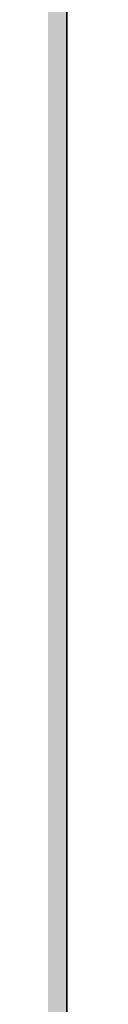
# Model space of a CAD drawing. Units: inches. Extents: x 2083 to 3317, y 1141 to 2115.
# Tile 170 of 256: x 3126.959687 to 3126.959831, y 1263.265937 to 1263.274018. Entities that reach past the tile are written whole.
import ezdxf

# ---------------------------------------------------------------- set-up
doc = ezdxf.new("R2010")
doc.units = ezdxf.units.IN
doc.layers.add('A-ANNO-DIMS', color=2, linetype='Continuous', lineweight=18)
doc.layers.add('A-WALL', color=7, linetype='Continuous', lineweight=35)
doc.layers.add('A-WALL-PATT', color=251, linetype='Continuous', lineweight=13, true_color=0x636466)
doc.styles.get("Standard").update_dxf_attribs({"font": 'arial.ttf'})
doc.dimstyles.new('ISO-25', dxfattribs={"dimtxt": 12, "dimasz": 12, "dimexe": 1.25, "dimexo": 0.625, "dimtad": 1, "dimlunit": 3, "dimtxsty": 'Standard', "dimcen": 2.5, "dimadec": 0, "dimazin": 0, "dimtfac": 1, "dimtmove": 0, "dimatfit": 3, "dimfxl": 1, "dimarcsym": 0})

# ---------------------------------------------------------------- blocks, each defined once
blk = doc.blocks.new('*D9')
at = {"layer": 'A-ANNO-DIMS', "color": 0, "lineweight": -2, "transparency": 16777216}
for p, q in [((3127.5847832, 1486.7613601), (3190.4030896, 1486.7613601)), ((3189.1530896, 1474.7613601), (3189.1530896, 1275.2613601)), ((3127.5847832, 1263.2613601), (3190.4030896, 1263.2613601))]:
    blk.add_line(p, q, dxfattribs=at)
at = {"layer": 'A-ANNO-DIMS', "color": 0, "transparency": 16777216}
for points in [[(3187.1530896, 1474.7613601), (3191.1530896, 1474.7613601), (3189.1530896, 1486.7613601)], [(3187.1530896, 1275.2613601), (3191.1530896, 1275.2613601), (3189.1530896, 1263.2613601)]]:
    blk.add_solid(points, dxfattribs=at)
at = {"layer": 'Defpoints', "color": 0, "transparency": 16777216}
for p in [(3126.9597832, 1486.7613601), (3126.9597832, 1263.2613601), (3189.1530896, 1263.2613601)]:
    blk.add_point(p, dxfattribs=at)
at = {"layer": 'A-ANNO-DIMS', "color": 0, "transparency": 16777216, "insert": (3182.4012138, 1375.0113601), "char_height": 12, "attachment_point": 5, "rotation": 90}
blk.add_mtext('18\'-7.5"', dxfattribs=at)

msp = doc.modelspace()

# ---------------------------------------------------------------- hatches: boundary and pattern name
at = {"layer": 'A-WALL-PATT'}
h = msp.add_hatch(color=256, dxfattribs=at)
h.dxf.hatch_style = 1
h.paths.add_polyline_path([(3126.9597832, 2020.7613601), (2748.9597832, 2020.7613601), (2604.9597832, 2020.7613601), (2226.9597832, 2020.7613601), (2226.9597832, 1702.7613601), (2466.9597832, 1702.7613601), (2466.9597832, 1582.7613601), (2418.9597832, 1582.7613601), (2418.9597832, 1477.7613601), (2226.9597832, 1477.7613601), (2226.9597832, 1263.2613601), (2544.9597832, 1263.2613601), (2544.9597832, 1411.7613601), (2604.9597832, 1411.7613601), (2685.9597832, 1411.7613601), (2685.9597832, 1420.7613601), (2604.9597832, 1420.7613601), (2604.9597832, 1573.7613601), (2604.9597832, 1702.7613601), (2604.9597832, 2011.7613601), (2748.9597832, 2011.7613601), (2748.9597832, 1702.7613601), (2862.9597832, 1702.7613601), (2862.9597832, 1621.7613601), (2871.9597832, 1621.7613601), (2871.9597832, 1702.7613601), (2883.9597832, 1702.7613601), (2883.9597832, 1706.9394595, -0.026459), (2883.9597832, 1711.7613601), (2757.9597832, 1711.7613601), (2757.9597832, 1807.7613601), (2787.9597832, 1807.7613601), (2787.9597832, 1812.2613601), (2757.9597832, 1812.2613601), (2757.9597832, 2011.7613601), (2877.9597832, 2011.7613601), (2877.9597832, 1812.2613601), (2847.9597832, 1812.2613601), (2847.9597832, 1807.7613601), (2889.8357425, 1807.7613601), (2889.8357425, 1812.2613601), (2882.4597832, 1812.2613601), (2882.4597832, 2011.7613601), (3117.9597832, 2011.7613601), (3117.9597832, 1812.2613601), (2937.8357425, 1812.2613601), (2937.8357425, 1807.7613601), (2995.7097832, 1807.7613601), (2995.7097832, 1796.1176655), (3000.2097832, 1796.1176655), (3000.2097832, 1807.7613601), (3117.9597832, 1807.7613601), (3117.9597832, 1711.7613601), (3000.2097832, 1711.7613601), (3000.2097832, 1760.1176655), (2998.5727047, 1760.1176655, -0.020711), (2995.7097832, 1760.1176655), (2995.7097832, 1711.7613601), (2931.9597832, 1711.7613601), (2931.9597832, 1702.7613601), (3126.9597832, 1702.7613601)])
h.paths.add_polyline_path([(2471.4597832, 2011.7613601), (2471.4597832, 1810.0113601), (2462.7169357, 1810.0113601), (2462.7169357, 1805.5113601), (2505.9597832, 1805.5113601), (2505.9597832, 1810.0113601), (2475.9597832, 1810.0113601), (2475.9597832, 2011.7613601), (2595.9597832, 2011.7613601), (2595.9597832, 1810.0113601), (2565.9597832, 1810.0113601), (2565.9597832, 1805.5113601), (2595.9597832, 1805.5113601), (2595.9597832, 1711.7613601), (2235.9597832, 1711.7613601), (2235.9597832, 1805.5113601), (2353.7097832, 1805.5113601), (2353.7097832, 1796.0541624), (2358.2097832, 1796.0541624), (2358.2097832, 1805.5113601), (2414.7169357, 1805.5113601), (2414.7169357, 1810.0113601), (2235.9597832, 1810.0113601), (2235.9597832, 2011.7613601)], flags=16)
h.paths.add_polyline_path([(2270.2047343, 1994.6100082), (2270.2047343, 1970.6100082), (2246.2047343, 1970.6100082), (2246.2047343, 1994.6100082)], flags=0)
edge = h.paths.add_edge_path(flags=0)
edge.add_ellipse((2332.027391, 1899.7981761), major_axis=(-3.0429938, 3.0429938), ratio=0.16825245, start_angle=-161.3321656, end_angle=-156.3071136, ccw=False)
edge.add_ellipse((2333.0820373, 1898.7435297), major_axis=(-1.0546463, 1.0546463), ratio=0.453532097, start_angle=-123.371019, end_angle=-94.1591066)
edge = h.paths.add_edge_path(flags=0)
edge.add_ellipse((2332.027391, 1968.8762897), major_axis=(3.0429938, 3.0429938), ratio=0.16825245, start_angle=18.6678344, end_angle=23.6928864)
edge.add_spline(control_points=[(2332.9255964, 1970.6911045), (2332.2267681, 1970.3360997), (2330.8937087, 1969.6589054), (2328.4130803, 1970.9321376), (2327.2039345, 1967.7487119), (2324.7095965, 1969.9555886), (2322.5328223, 1967.012354), (2320.0128462, 1971.2958124), (2317.6803077, 1968.1578449), (2316.0405263, 1967.1020468), (2315.4269045, 1966.8096022)], knot_values=[0, 0, 0, 0, 2.267059, 4.324559, 6.685584, 8.878641, 11.121502, 14.300359, 17.755284, 19.732645, 19.732645, 19.732645, 19.732645], degree=3, periodic=0)
edge.add_ellipse((2332.027391, 1968.8762897), major_axis=(3.0429938, 3.0429938), ratio=0.16825245, start_angle=18.6678344, end_angle=23.6928864, ccw=False)
edge.add_ellipse((2333.0820373, 1969.930936), major_axis=(1.0546463, 1.0546463), ratio=0.453532097, start_angle=56.628981, end_angle=85.8408934, ccw=False)
edge = h.paths.add_edge_path(flags=0)
edge.add_spline(control_points=[(2296.4282874, 1967.9879081), (2293.6278045, 1965.3363137), (2287.7036238, 1959.727094), (2299.7438601, 1949.9956993), (2294.5325909, 1935.6685275), (2290.5732281, 1920.6035119), (2293.3941244, 1909.9736911), (2296.1854073, 1904.9665431)], knot_values=[0.099185, 0.099185, 0.099185, 0.099185, 0.345301, 0.619822, 0.982653, 1.386093, 1.810555, 1.810555, 1.810555, 1.810555], degree=3, periodic=0)
edge.add_spline(control_points=[(2296.1854073, 1904.9665431), (2297.3835817, 1902.6193002), (2298.0009694, 1901.9493116), (2298.5529698, 1901.4681549)], knot_values=[0.006246, 0.006246, 0.006246, 0.006246, 0.055476, 0.055476, 0.055476, 0.055476], degree=3, periodic=0)
edge.add_spline(control_points=[(2298.5529698, 1901.4681549), (2297.2586121, 1900.9232238), (2295.2252939, 1900.2321257), (2293.0602287, 1900.6142053), (2292.1014227, 1900.788415), (2292.0895776, 1900.790568)], knot_values=[0.312835, 0.312835, 0.312835, 0.312835, 0.40178, 0.474987, 0.475903, 0.475903, 0.475903, 0.475903], degree=3, periodic=0)
edge.add_arc((2292.7936464, 1904.6641088), 3.9370079, 215.4208969, 259.6981795, ccw=False)
edge.add_spline(control_points=[(2289.5853139, 1902.3823039), (2289.4766524, 1902.5350874), (2289.3684805, 1902.6880353), (2289.2608648, 1902.8411699)], knot_values=[0.102872, 0.102872, 0.102872, 0.102872, 0.116896, 0.116896, 0.116896, 0.116896], degree=3, periodic=0)
edge.add_spline(control_points=[(2289.2608648, 1902.8411699), (2288.6866042, 1902.5501922), (2287.6400477, 1902.0199025), (2285.8813368, 1901.8739536), (2283.8529717, 1901.5043521), (2281.7199871, 1899.7105375), (2278.4669913, 1899.492942), (2276.1571361, 1901.8832022), (2272.2589526, 1899.8040711), (2267.7776054, 1901.8431828), (2262.2438819, 1900.1840326), (2257.414927, 1901.7820606), (2254.318374, 1900.7261196), (2253.1782849, 1900.3373431)], knot_values=[0, 0, 0, 0, 1.907977, 3.477176, 5.261074, 7.972851, 11.680248, 13.717921, 16.939592, 22.789562, 27.502503, 33.595215, 37.145618, 37.145618, 37.145618, 37.145618], degree=3, periodic=0)
edge.add_line((2253.1782849, 1900.3373431), (2250.2442397, 1902.8411699))
edge.add_line((2250.2442397, 1902.8411699), (2250.2442397, 1965.8332959))
edge.add_line((2250.2442397, 1965.8332959), (2253.1782849, 1968.3371226))
edge.add_spline(control_points=[(2253.1782849, 1968.3371226), (2254.318374, 1967.9483462), (2257.414927, 1966.8924051), (2262.2438819, 1968.4904332), (2267.7776054, 1966.8312829), (2271.5267301, 1968.5372172), (2273.8759143, 1967.8282895), (2274.2067012, 1967.7276424)], knot_values=[0, 0, 0, 0, 0.09018, 0.244935, 0.364644, 0.513233, 0.537855, 0.537855, 0.537855, 0.537855], degree=3, periodic=0)
edge.add_arc((2274.3528869, 1963.7933495), 3.9370079, 72.0511336, 92.1279492, ccw=False)
edge.add_arc((2281.2969331, 1985.2300027), 18.5962982, 252.05113361, 288.56572166)
edge.add_arc((2292.3167172, 1956.0288805), 12.6460805, 71.02678788, 113.77821843, ccw=False)
edge = h.paths.add_edge_path(flags=0)
edge.add_spline(control_points=[(2274.8994147, 1951.8561946), (2275.066156, 1951.6165924), (2275.2326866, 1951.3765878), (2275.3979871, 1951.1358545)], knot_values=[1.409916, 1.409916, 1.409916, 1.409916, 1.43159, 1.43159, 1.43159, 1.43159], degree=3, periodic=0)
edge.add_spline(control_points=[(2275.3979871, 1951.1358545), (2275.7921055, 1950.5618854), (2276.1792311, 1949.9837745), (2276.5455462, 1949.3971029)], knot_values=[1.358238, 1.358238, 1.358238, 1.358238, 1.409916, 1.409916, 1.409916, 1.409916], degree=3, periodic=0)
edge.add_line((2276.5455462, 1949.3971029), (2277.437289, 1947.8621847))
edge.add_spline(control_points=[(2277.437289, 1947.8621847), (2276.3038341, 1945.6731147), (2274.6396979, 1942.4268817), (2274.631615, 1938.0938998), (2272.7991237, 1930.8515498), (2274.3564261, 1943.8970461), (2275.9476814, 1947.9233558), (2276.5455462, 1949.3971029)], knot_values=[0.005632, 0.005632, 0.005632, 0.005632, 0.186014, 0.266002, 0.357087, 0.59639, 0.739732, 0.739732, 0.739732, 0.739732], degree=3, periodic=0)
edge.add_spline(control_points=[(2276.5455462, 1949.3971029), (2276.1792311, 1949.9837745), (2275.7921055, 1950.5618854), (2275.3979871, 1951.1358545)], knot_values=[1.358238, 1.358238, 1.358238, 1.358238, 1.409916, 1.409916, 1.409916, 1.409916], degree=3, periodic=0)
edge.add_spline(control_points=[(2275.3979871, 1951.1358545), (2274.9425002, 1950.0804523), (2274.2077604, 1948.0252718), (2273.9346018, 1944.8514774), (2272.4685341, 1937.6274891), (2273.4662155, 1945.6964663), (2274.7006154, 1951.0594725), (2274.8994147, 1951.8561946)], knot_values=[0.104364, 0.104364, 0.104364, 0.104364, 0.189636, 0.269624, 0.36071, 0.600013, 0.644622, 0.644622, 0.644622, 0.644622], degree=3, periodic=0)
h.paths.add_polyline_path([(2269.1675139, 1963.1275729, -0.357527), (2268.170633, 1960.9763695, -0.092561), (2268.170633, 1939.4363249, -0.357527), (2269.1675139, 1937.2851215, -0.357527), (2267.0163105, 1938.2820024, -0.164785), (2254.6855813, 1938.2820024, -0.357527), (2252.5343779, 1937.2851215, -0.357527), (2253.5312587, 1939.4363249, -0.092561), (2253.5312587, 1960.9763695, -0.357527), (2252.5343779, 1963.1275729, -0.357527), (2254.6855813, 1962.130692, -0.164785), (2267.0163105, 1962.130692, -0.357527)], flags=0)
h.paths.add_polyline_path([(2248.8740679, 1967.8017998), (2248.8740679, 1957.0277095), (2249.4577833, 1957.0277095), (2249.4577833, 1911.6467562), (2248.8740679, 1911.6467562), (2248.8740679, 1900.8726659), (2246.5118632, 1900.8726659, 0.197327), (2244.1496584, 1902.4568734), (2244.1496584, 1966.2175923, 0.197327), (2246.5118632, 1967.8017998)], flags=0)
h.paths.add_polyline_path([(2269.1675139, 1931.3893442, -0.357527), (2268.170633, 1929.2381408, -0.092561), (2268.170633, 1907.6980962, -0.357527), (2269.1675139, 1905.5468928, -0.357527), (2267.0163105, 1906.5437737, -0.164785), (2254.6855813, 1906.5437737, -0.357527), (2252.5343779, 1905.5468928, -0.357527), (2253.5312587, 1907.6980962, -0.092561), (2253.5312587, 1929.2381408, -0.357527), (2252.5343779, 1931.3893442, -0.357527), (2254.6855813, 1930.3924634, -0.164785), (2267.0163105, 1930.3924634, -0.357527)], flags=0)
edge = h.paths.add_edge_path(flags=0)
edge.add_spline(control_points=[(2276.1968578, 1906.7237016), (2276.1681442, 1909.0289278), (2276.1140492, 1913.371852), (2270.5984171, 1924.9249783), (2273.9051746, 1919.0127787), (2275.9217115, 1916.2620626), (2275.4745699, 1912.4021495), (2277.2578735, 1910.3806206), (2276.6960436, 1908.2250358), (2276.6462176, 1906.8130226), (2276.6178249, 1906.0084068)], knot_values=[0, 0, 0, 0, 8.61026, 16.221274, 18.843057, 23.804898, 27.440828, 29.356102, 31.203478, 33.650687, 33.650687, 33.650687, 33.650687], degree=3, periodic=0)
edge.add_spline(control_points=[(2276.6178249, 1906.0084068), (2276.6233131, 1905.6241436), (2276.4977381, 1904.6286608), (2275.4417789, 1903.8547251), (2274.9373144, 1903.0804497), (2274.8590804, 1902.8411699)], knot_values=[0.156488, 0.156488, 0.156488, 0.156488, 0.184398, 0.231376, 0.250598, 0.250598, 0.250598, 0.250598], degree=3, periodic=0)
edge.add_line((2274.8590804, 1902.8411699), (2276.50598, 1902.8411699))
edge.add_spline(control_points=[(2276.50598, 1902.8411699), (2276.7883084, 1903.0849395), (2277.6650711, 1904.1251958), (2278.2495378, 1904.340738), (2277.6538719, 1908.5273866), (2278.15567, 1906.2278078), (2278.100464, 1905.2859484), (2278.8466748, 1904.0690054), (2277.8567853, 1903.4149482), (2277.8741909, 1902.9910497), (2277.9035616, 1902.8411699)], knot_values=[0.059574, 0.059574, 0.059574, 0.059574, 0.080753, 0.103741, 0.16972, 0.176036, 0.207137, 0.240474, 0.262341, 0.27366, 0.27366, 0.27366, 0.27366], degree=3, periodic=0)
edge.add_line((2277.9035616, 1902.8411699), (2280.0298255, 1902.8411699))
edge.add_spline(control_points=[(2280.0298255, 1902.8411699), (2279.8882214, 1903.088398), (2279.4992571, 1903.9815512), (2280.1522839, 1905.9393491), (2278.103615, 1909.6577572), (2279.7623946, 1907.185285), (2280.3279002, 1904.8748608), (2280.4851086, 1903.4895904), (2281.4632687, 1903.2494323), (2281.7583431, 1902.9364967), (2281.8340361, 1902.8411699)], knot_values=[0.013856, 0.013856, 0.013856, 0.013856, 0.034874, 0.088867, 0.107879, 0.126738, 0.158714, 0.193757, 0.217487, 0.226722, 0.226722, 0.226722, 0.226722], degree=3, periodic=0)
edge.add_spline(control_points=[(2281.8340361, 1902.8411699), (2281.7875348, 1902.8267029), (2281.6470224, 1902.7829881), (2281.3955272, 1902.85949), (2281.088077, 1902.9852418), (2280.7206826, 1903.060902), (2280.3334513, 1903.0257257), (2280.1247668, 1902.898879), (2280.0298255, 1902.8411699)], knot_values=[0, 0, 0, 0, 0.14413, 0.435517, 0.749276, 1.153046, 1.548371, 1.878348, 1.878348, 1.878348, 1.878348], degree=3, periodic=0)
edge.add_line((2280.0298255, 1902.8411699), (2277.9035616, 1902.8411699))
edge.add_spline(control_points=[(2277.9035616, 1902.8411699), (2277.892855, 1902.7958553), (2277.865396, 1902.6796374), (2277.6074793, 1902.6874828), (2277.2740503, 1902.8006999), (2276.8379209, 1902.6197745), (2276.5838074, 1902.7892611), (2276.50598, 1902.8411699)], knot_values=[0, 0, 0, 0, 0.127189, 0.326199, 0.628009, 1.24357, 1.515331, 1.515331, 1.515331, 1.515331], degree=3, periodic=0)
edge.add_line((2276.50598, 1902.8411699), (2274.8590804, 1902.8411699))
edge.add_spline(control_points=[(2274.8590804, 1902.8411699), (2274.8144367, 1902.8985868), (2274.7251297, 1903.013446), (2274.4934765, 1903.1189684), (2274.2442854, 1902.9605386), (2273.9371207, 1903.1849416), (2273.6140395, 1902.9831428), (2273.4083164, 1902.8830449), (2273.322254, 1902.8411699)], knot_values=[0, 0, 0, 0, 0.21843, 0.436957, 0.687977, 0.990379, 1.398396, 1.69185, 1.69185, 1.69185, 1.69185], degree=3, periodic=0)
edge.add_spline(control_points=[(2273.322254, 1902.8411699), (2273.6167403, 1903.445692), (2274.2739977, 1904.5382529), (2276.0272387, 1904.5737017), (2276.2069634, 1906.5836372), (2276.1968578, 1906.7237016)], knot_values=[0.012227, 0.012227, 0.012227, 0.012227, 0.059472, 0.106218, 0.134458, 0.134458, 0.134458, 0.134458], degree=3, periodic=0)
h.paths.add_polyline_path([(2270.7760538, 1897.7898284), (2270.7760538, 1873.7898284), (2246.7760538, 1873.7898284), (2246.7760538, 1897.7898284)], flags=0)
h.paths.add_polyline_path([(2353.7097832, 1760.0050593), (2353.7097832, 1760.0541624), (2358.2097832, 1760.0541624, -0.033729)], flags=0)
h.paths.add_polyline_path([(2321.8191188, 1737.5291862), (2341.9953271, 1737.5291862, -0.414214), (2343.2032727, 1736.3212406), (2343.2032727, 1721.0205964, -0.414214), (2341.9953271, 1719.8126508), (2321.8191188, 1719.8126508, -0.414214), (2320.6111732, 1721.0205964), (2320.6111732, 1736.3212406, -0.414214)], flags=0)
h.paths.add_polyline_path([(2324.2350099, 1736.3212406), (2339.5794359, 1736.3212406, -0.414214), (2341.9953271, 1733.9053494), (2341.9953271, 1725.4497302, -0.414214), (2339.5794359, 1723.033839), (2333.6805885, 1723.033839), (2333.8453172, 1722.0454666, -0.870646), (2335.4253988, 1721.8258934, -0.767327), (2333.922694, 1721.4232449), (2331.2910241, 1721.4232449, -0.767327), (2329.7883193, 1721.8258934, -0.870646), (2331.3684009, 1722.0454666), (2331.5331296, 1723.033839), (2324.2350099, 1723.033839, -0.414214), (2321.8191188, 1725.4497302), (2321.8191188, 1733.9053494, -0.414214)], flags=0)
h.paths.add_polyline_path([(2570.4837892, 1928.6154443), (2589.6837892, 1928.6154443), (2590.1688286, 1928.6154443), (2590.1688286, 1904.9933971), (2570.4837892, 1904.9933971)], flags=0)
h.paths.add_polyline_path([(2574.4473242, 1927.2638215, -1), (2572.8288357, 1927.2638215, -1)], flags=0)
h.paths.add_polyline_path([(2573.0898665, 1926.9408768), (2573.925032, 1927.7760423), (2574.1477428, 1927.5533315), (2573.3125773, 1926.718166)], flags=0)
h.paths.add_polyline_path([(2578.7790648, 1919.7296175, -1), (2571.5916632, 1919.7296175, -1)], flags=0)
h.paths.add_polyline_path([(2578.385364, 1919.7296175, -1), (2571.985364, 1919.7296175, -1)], flags=0)
h.paths.add_polyline_path([(2331.5957638, 1729.4762156, -1), (2333.6179542, 1729.4762156, -1)], flags=0)
h.paths.add_polyline_path([(2578.0342282, 1927.2638215, -1), (2576.4157396, 1927.2638215, -1)], flags=0)
h.paths.add_polyline_path([(2576.6888513, 1927.5310886), (2576.9115621, 1927.7537993), (2577.7467276, 1926.9186339), (2577.5240168, 1926.6959231)], flags=0)
h.paths.add_polyline_path([(2578.1390648, 1909.8595388, -1), (2572.2316632, 1909.8595388, -1)], flags=0)
h.paths.add_polyline_path([(2577.745364, 1909.8595388, -1), (2572.625364, 1909.8595388, -1)], flags=0)
h.paths.add_polyline_path([(2583.7977179, 1927.2638215, -1), (2582.1792294, 1927.2638215, -1)], flags=0)
h.paths.add_polyline_path([(2582.7186487, 1927.7537993), (2583.5538142, 1926.9186339), (2583.3311034, 1926.6959231), (2582.4959379, 1927.5310886)], flags=0)
h.paths.add_polyline_path([(2582.4959379, 1927.5310886), (2582.7186487, 1927.7537993), (2583.5538142, 1926.9186339), (2583.3311034, 1926.6959231)], flags=0)
h.paths.add_polyline_path([(2587.7390648, 1920.5296175, -1), (2581.8316632, 1920.5296175, -1)], flags=0)
h.paths.add_polyline_path([(2587.345364, 1920.5296175, -1), (2582.225364, 1920.5296175, -1)], flags=0)
h.paths.add_polyline_path([(2587.3846219, 1927.2638215, -1), (2585.7661333, 1927.2638215, -1)], flags=0)
h.paths.add_polyline_path([(2586.0819925, 1926.9802469), (2586.917158, 1927.8154124), (2587.1398688, 1927.5927016), (2586.3047033, 1926.7575361)], flags=0)
h.paths.add_polyline_path([(2588.3790648, 1910.6595388, -1), (2581.1916632, 1910.6595388, -1)], flags=0)
h.paths.add_polyline_path([(2587.985364, 1910.6595388, -1), (2581.585364, 1910.6595388, -1)], flags=0)
h.paths.add_polyline_path([(2417.1677288, 1729.4778955), (2437.3439372, 1729.4778955, -0.414214), (2438.5518828, 1728.2699499), (2438.5518828, 1712.9693057, -0.414214), (2437.3439372, 1711.7613601), (2417.1677288, 1711.7613601, -0.414214), (2415.9597832, 1712.9693057), (2415.9597832, 1728.2699499, -0.414214)], flags=0)
h.paths.add_polyline_path([(2419.58362, 1728.2699499), (2434.928046, 1728.2699499, -0.414214), (2437.3439372, 1725.8540587), (2437.3439372, 1717.3984395, -0.414214), (2434.928046, 1714.9825483), (2429.0291985, 1714.9825483), (2429.1939273, 1713.9941758, -0.870646), (2430.7740089, 1713.7746027, -0.767327), (2429.2713041, 1713.3719542), (2426.6396342, 1713.3719542, -0.767327), (2425.1369294, 1713.7746027, -0.870646), (2426.717011, 1713.9941758), (2426.8817397, 1714.9825483), (2419.58362, 1714.9825483, -0.414214), (2417.1677288, 1717.3984395), (2417.1677288, 1725.8540587, -0.414214)], flags=0)
h.paths.add_polyline_path([(2419.58362, 1728.2699499), (2434.928046, 1728.2699499, -0.414214), (2437.3439372, 1725.8540587), (2437.3439372, 1717.3984395, -0.414214), (2434.928046, 1714.9825483), (2429.0291985, 1714.9825483), (2428.3581177, 1719.0090337), (2427.5528206, 1719.0090337), (2426.8817397, 1714.9825483), (2419.58362, 1714.9825483, -0.414214), (2417.1677288, 1717.3984395), (2417.1677288, 1725.8540587, -0.414214)], flags=0)
h.paths.add_polyline_path([(2426.9443739, 1721.4249248, -1), (2428.9665643, 1721.4249248, -1)], flags=0)
h.paths.add_polyline_path([(2475.9597832, 1702.7613601), (2595.9597832, 1702.7613601), (2595.9597832, 1582.7613601), (2475.9597832, 1582.7613601)], flags=16)
h.paths.add_polyline_path([(2427.9597832, 1573.7613601), (2595.9597832, 1573.7613601), (2595.9597832, 1468.7613601), (2595.9597832, 1420.7613601), (2384.4597832, 1420.7613601), (2384.4597832, 1468.7613601), (2427.9597832, 1468.7613601)], flags=16)
h.paths.add_polyline_path([(2379.9597832, 1468.7613601), (2379.9597832, 1420.7613601), (2235.9597832, 1420.7613601), (2235.9597832, 1468.7613601)], flags=16)
h.paths.add_polyline_path([(2317.8159962, 1466.695767), (2337.9922045, 1466.695767, -0.414214), (2339.2001501, 1465.4878214), (2339.2001501, 1450.1871771, -0.414214), (2337.9922045, 1448.9792315), (2317.8159962, 1448.9792315, -0.414214), (2316.6080506, 1450.1871771), (2316.6080506, 1465.4878214, -0.414214)], flags=0)
h.paths.add_polyline_path([(2320.2318874, 1465.4878214), (2335.5763133, 1465.4878214, -0.414214), (2337.9922045, 1463.0719302), (2337.9922045, 1454.616311, -0.414214), (2335.5763133, 1452.2004198), (2329.6774659, 1452.2004198), (2329.8421946, 1451.2120473, -0.870646), (2331.4222762, 1450.9924742, -0.767327), (2329.9195714, 1450.5898257), (2327.2879015, 1450.5898257, -0.767327), (2325.7851967, 1450.9924742, -0.870646), (2327.3652783, 1451.2120473), (2327.530007, 1452.2004198), (2320.2318874, 1452.2004198, -0.414214), (2317.8159962, 1454.616311), (2317.8159962, 1463.0719302, -0.414214)], flags=0)
h.paths.add_polyline_path([(2320.2318874, 1465.4878214), (2335.5763133, 1465.4878214, -0.414214), (2337.9922045, 1463.0719302), (2337.9922045, 1454.616311, -0.414214), (2335.5763133, 1452.2004198), (2329.6774659, 1452.2004198), (2329.006385, 1456.2269051), (2328.2010879, 1456.2269051), (2327.530007, 1452.2004198), (2320.2318874, 1452.2004198, -0.414214), (2317.8159962, 1454.616311), (2317.8159962, 1463.0719302, -0.414214)], flags=0)
h.paths.add_polyline_path([(2327.5926413, 1458.6427963, -1), (2329.6148317, 1458.6427963, -1)], flags=0)
h.paths.add_polyline_path([(2244.4117436, 1433.3404531), (2241.9209449, 1433.3404531, -0.414214), (2240.0178562, 1435.2435418), (2240.0178562, 1440.9528078, -0.414211), (2241.920925, 1442.8558965), (2244.4117436, 1442.8558965, -1.976472)], flags=0)
h.paths.add_polyline_path([(2245.3568884, 1434.3975358, -0.414214), (2245.3568884, 1441.7988138, -2.144098)], flags=0)
h.paths.add_polyline_path([(2535.9597832, 1416.2613601), (2535.9597832, 1272.2613601), (2235.9597832, 1272.2613601), (2235.9597832, 1416.2613601)], flags=16)
h.paths.add_polyline_path([(2260.1195614, 1384.2928413), (2260.1195614, 1362.0386487), (2237.8653688, 1362.0386487), (2237.8653688, 1384.2928413)], flags=0)
edge = h.paths.add_edge_path(flags=0)
edge.add_line((2318.2518466, 1362.0932983), (2318.1457968, 1362.0009726))
edge.add_ellipse((2317.4451158, 1360.4310442), major_axis=(2.8216404, 2.8216404), ratio=0.16825245, start_angle=18.6678344, end_angle=20.9481273, ccw=False)
edge.add_ellipse((2318.4230451, 1361.4089735), major_axis=(0.9779293, 0.9779293), ratio=0.453532097, start_angle=56.628981, end_angle=70.2262012, ccw=False)
edge = h.paths.add_edge_path(flags=0)
edge.add_line((2319.1073699, 1295.5710784), (2319.0150442, 1295.6771282))
edge.add_ellipse((2317.4451158, 1296.3778091), major_axis=(-2.8216404, 2.8216404), ratio=0.16825245, start_angle=-161.3321656, end_angle=-159.0518727, ccw=False)
edge.add_ellipse((2318.4230451, 1295.3998798), major_axis=(-0.9779293, 0.9779293), ratio=0.453532097, start_angle=-123.371019, end_angle=-109.7737988)
edge = h.paths.add_edge_path(flags=0)
edge.add_spline(control_points=[(2284.2103489, 1301.1702189), (2284.5806878, 1300.444719), (2284.8911891, 1299.8920243), (2285.159553, 1299.4610182)], knot_values=[0.039066, 0.039066, 0.039066, 0.039066, 0.055476, 0.055476, 0.055476, 0.055476], degree=3, periodic=0)
edge.add_line((2285.159553, 1299.4610182), (2284.2103489, 1301.1702189))
edge = h.paths.add_edge_path(flags=0)
edge.add_line((2280.4124579, 1297.2980125), (2283.3699905, 1297.0361216))
edge.add_line((2283.3699905, 1297.0361216), (2286.4056902, 1297.9263104))
edge.add_spline(control_points=[(2286.4056902, 1297.9263104), (2285.305487, 1297.4631193), (2284.3447774, 1297.1291508), (2283.3699905, 1297.0361216)], knot_values=[0.394369, 0.394369, 0.394369, 0.394369, 0.475903, 0.475903, 0.475903, 0.475903], degree=3, periodic=0)
edge.add_spline(control_points=[(2283.3699905, 1297.0361216), (2283.2813895, 1297.027666), (2282.316289, 1296.9573356), (2281.3125019, 1297.1344787), (2280.4234414, 1297.2960161), (2280.4124579, 1297.2980125)], knot_values=[0.312835, 0.312835, 0.312835, 0.312835, 0.320246, 0.393453, 0.394369, 0.394369, 0.394369, 0.394369], degree=3, periodic=0)
edge = h.paths.add_edge_path(flags=0)
edge.add_line((2284.4355615, 1359.6072854), (2280.4462909, 1355.328047))
edge.add_line((2280.4462909, 1355.328047), (2279.5799868, 1351.0177544))
edge.add_line((2279.5799868, 1351.0177544), (2282.4129737, 1346.5804327))
edge.add_spline(control_points=[(2282.4129737, 1346.5804327), (2283.1533308, 1345.5892358), (2284.2528957, 1344.0288973), (2284.801037, 1342.3871671), (2284.9351625, 1341.8055443)], knot_values=[1.240098, 1.240098, 1.240098, 1.240098, 1.332892, 1.382712, 1.382712, 1.382712, 1.382712], degree=3, periodic=0)
edge.add_spline(control_points=[(2284.9351625, 1341.8055443), (2285.3191079, 1340.1406002), (2285.2330291, 1338.4092041), (2284.9099384, 1336.6541222)], knot_values=[1.097484, 1.097484, 1.097484, 1.097484, 1.240098, 1.240098, 1.240098, 1.240098], degree=3, periodic=0)
edge.add_spline(control_points=[(2284.9099384, 1336.6541222), (2284.5868478, 1334.8990403), (2284.0267453, 1333.1202725), (2283.4626437, 1331.3605849)], knot_values=[0.95487, 0.95487, 0.95487, 0.95487, 1.097484, 1.097484, 1.097484, 1.097484], degree=3, periodic=0)
edge.add_line((2283.4626437, 1331.3605849), (2281.8903759, 1326.153357))
edge.add_line((2281.8903759, 1326.153357), (2280.7562592, 1321.0560888))
edge.add_line((2280.7562592, 1321.0560888), (2280.2992048, 1316.0019772))
edge.add_line((2280.2992048, 1316.0019772), (2280.7159327, 1310.9500678))
edge.add_line((2280.7159327, 1310.9500678), (2282.0280939, 1305.9721367))
edge.add_line((2282.0280939, 1305.9721367), (2284.2103489, 1301.1702189))
edge.add_spline(control_points=[(2284.2103489, 1301.1702189), (2283.3407305, 1302.7301854), (2282.6119044, 1304.3364933), (2282.0280939, 1305.9721367)], knot_values=[0.099185, 0.099185, 0.099185, 0.099185, 0.241799, 0.241799, 0.241799, 0.241799], degree=3, periodic=0)
edge.add_spline(control_points=[(2282.0280939, 1305.9721367), (2281.4442835, 1307.6077801), (2281.0054886, 1309.2727591), (2280.7159327, 1310.9500678)], knot_values=[0.241799, 0.241799, 0.241799, 0.241799, 0.384413, 0.384413, 0.384413, 0.384413], degree=3, periodic=0)
edge.add_spline(control_points=[(2280.7159327, 1310.9500678), (2280.4332411, 1312.5876134), (2280.2893863, 1314.2769594), (2280.2988938, 1315.9620324), (2280.2992048, 1316.0019772)], knot_values=[0.384413, 0.384413, 0.384413, 0.384413, 0.523647, 0.527028, 0.527028, 0.527028, 0.527028], degree=3, periodic=0)
edge.add_spline(control_points=[(2280.2992048, 1316.0019772), (2280.3123257, 1317.6869552), (2280.4778706, 1319.3679256), (2280.7562592, 1321.0560888)], knot_values=[0.527028, 0.527028, 0.527028, 0.527028, 0.669642, 0.669642, 0.669642, 0.669642], degree=3, periodic=0)
edge.add_spline(control_points=[(2280.7562592, 1321.0560888), (2281.0346478, 1322.7442519), (2281.4258801, 1324.4396079), (2281.8903759, 1326.153357)], knot_values=[0.669642, 0.669642, 0.669642, 0.669642, 0.812256, 0.812256, 0.812256, 0.812256], degree=3, periodic=0)
edge.add_spline(control_points=[(2281.8903759, 1326.153357), (2282.2643834, 1327.5332507), (2282.7878702, 1329.2618097), (2283.352751, 1331.0177803), (2283.4626437, 1331.3605849)], knot_values=[0.812256, 0.812256, 0.812256, 0.812256, 0.927087, 0.95487, 0.95487, 0.95487, 0.95487], degree=3, periodic=0)
edge.add_line((2283.4626437, 1331.3605849), (2284.9099384, 1336.6541222))
edge.add_line((2284.9099384, 1336.6541222), (2284.9351625, 1341.8055443))
edge.add_line((2284.9351625, 1341.8055443), (2282.4129737, 1346.5804327))
edge.add_spline(control_points=[(2282.4129737, 1346.5804327), (2281.2751273, 1348.1037918), (2280.0784467, 1349.5703178), (2279.5799868, 1351.0177544)], knot_values=[1.382712, 1.382712, 1.382712, 1.382712, 1.525326, 1.525326, 1.525326, 1.525326], degree=3, periodic=0)
edge.add_spline(control_points=[(2279.5799868, 1351.0177544), (2279.4432818, 1351.4147209), (2279.1363124, 1352.856922), (2279.7351897, 1354.2903851), (2280.4462909, 1355.328047)], knot_values=[1.525326, 1.525326, 1.525326, 1.525326, 1.564439, 1.667941, 1.667941, 1.667941, 1.667941], degree=3, periodic=0)
edge.add_spline(control_points=[(2280.4462909, 1355.328047), (2281.4261132, 1356.7578354), (2282.9308373, 1358.1825604), (2284.4355615, 1359.6072854)], knot_values=[1.667941, 1.667941, 1.667941, 1.667941, 1.810555, 1.810555, 1.810555, 1.810555], degree=3, periodic=0)
edge.add_arc((2280.6230749, 1348.518181), 11.7261796, 71.02678788, 113.77821843)
edge.add_arc((2270.4048917, 1375.5951559), 17.2435667, 252.05113361, 288.56572166, ccw=False)
edge.add_arc((2263.9659692, 1355.7178471), 3.6506221, 72.0511336, 92.1279492)
edge.add_arc((2263.9659692, 1355.7178471), 3.6506221, 92.1279492, 177.98513)
edge.add_spline(control_points=[(2260.3176041, 1355.8461989), (2260.2604169, 1354.2206683), (2260.551278, 1350.1865469), (2262.9993445, 1346.7662507), (2264.4727415, 1344.6490245)], knot_values=[1.43159, 1.43159, 1.43159, 1.43159, 1.564144, 1.770695, 1.770695, 1.770695, 1.770695], degree=3, periodic=0)
edge.add_line((2264.4727415, 1344.6490245), (2264.9355904, 1343.9825301))
edge.add_spline(control_points=[(2263.8010444, 1340.2481052), (2263.8432379, 1340.5140884), (2264.0672444, 1341.7564652), (2264.5126928, 1343.0024532), (2264.9350468, 1343.9810834)], knot_values=[0.53657, 0.53657, 0.53657, 0.53657, 0.559349, 0.644622, 0.644622, 0.644622, 0.644622], degree=3, periodic=0)
edge.add_spline(control_points=[(2264.9350468, 1343.9810834), (2265.1177715, 1343.7149747), (2265.2988751, 1343.4479058), (2265.4767562, 1343.1793646)], knot_values=[1.384077, 1.384077, 1.384077, 1.384077, 1.409916, 1.409916, 1.409916, 1.409916], degree=3, periodic=0)
edge.add_spline(control_points=[(2265.4767562, 1343.1793646), (2265.6546373, 1342.9108234), (2265.8292958, 1342.64081), (2265.9991301, 1342.368812)], knot_values=[1.358238, 1.358238, 1.358238, 1.358238, 1.384077, 1.384077, 1.384077, 1.384077], degree=3, periodic=0)
edge.add_line((2265.9991301, 1342.368812), (2266.8260057, 1340.9455468))
edge.add_spline(control_points=[(2266.8260057, 1340.9455468), (2268.894401, 1337.0896912), (2271.3981727, 1325.8430009), (2270.5161644, 1310.5685568), (2275.9193759, 1301.860609), (2277.7895113, 1299.1994495)], knot_values=[0.116896, 0.116896, 0.116896, 0.116896, 0.472987, 1.050969, 1.313793, 1.313793, 1.313793, 1.313793], degree=3, periodic=0)
edge.add_spline(control_points=[(2277.7895113, 1299.1994495), (2277.8394051, 1299.1284519), (2277.8894277, 1299.0574975), (2277.9395717, 1298.9865839)], knot_values=[0.109884, 0.109884, 0.109884, 0.109884, 0.116896, 0.116896, 0.116896, 0.116896], degree=3, periodic=0)
edge.add_line((2277.9395717, 1298.9865839), (2277.7888489, 1299.1991139))
edge.add_spline(control_points=[(2277.7888489, 1299.1991139), (2277.2565819, 1298.9294144), (2276.2863504, 1298.4379024), (2275.0393517, 1298.3344186), (2274.3833299, 1298.2388951), (2274.2152543, 1298.209338)], knot_values=[33.12187, 33.12187, 33.12187, 33.12187, 35.029056, 36.598255, 37.144827, 37.144827, 37.144827, 37.144827], degree=3, periodic=0)
edge.add_line((2274.2152543, 1298.209338), (2273.073147, 1297.8929607))
edge.add_spline(control_points=[(2273.073147, 1297.8929607), (2272.3229363, 1297.579784), (2271.0391507, 1296.5105078), (2269.2483948, 1296.2260622), (2268.4231004, 1296.3746543)], knot_values=[26.532584, 26.532584, 26.532584, 26.532584, 29.198919, 31.839101, 31.839101, 31.839101, 31.839101], degree=3, periodic=0)
edge.add_line((2268.4231004, 1296.3746543), (2263.8785014, 1297.4575338))
edge.add_spline(control_points=[(2263.8785014, 1297.4575338), (2263.5560769, 1297.3594345), (2261.8603064, 1296.8386943), (2260.2387805, 1297.2824073), (2258.9334543, 1297.5164611)], knot_values=[15.919551, 15.919551, 15.919551, 15.919551, 16.939592, 21.226067, 21.226067, 21.226067, 21.226067], degree=3, periodic=0)
edge.add_line((2258.9334543, 1297.5164611), (2254.0552332, 1297.3290098))
edge.add_spline(control_points=[(2254.0552332, 1297.3290098), (2253.7555255, 1297.295815), (2252.1136834, 1297.1651738), (2250.4618687, 1297.5442209), (2249.1296862, 1297.6678818)], knot_values=[5.306517, 5.306517, 5.306517, 5.306517, 6.276435, 10.613034, 10.613034, 10.613034, 10.613034], degree=3, periodic=0)
edge.add_line((2249.1296862, 1297.6678818), (2244.3316495, 1296.8777561))
edge.add_line((2244.3316495, 1296.8777561), (2241.6110326, 1299.1994495))
edge.add_line((2241.6110326, 1299.1994495), (2241.6110326, 1357.6094038))
edge.add_line((2241.6110326, 1357.6094038), (2244.3316495, 1359.9310973))
edge.add_line((2244.3316495, 1359.9310973), (2252.7288228, 1359.5426917))
edge.add_spline(control_points=[(2252.7288228, 1359.5426917), (2252.8709387, 1359.5464396), (2253.3057402, 1359.5481716), (2253.7398447, 1359.5142744), (2254.0317419, 1359.4824261)], knot_values=[0.233291, 0.233291, 0.233291, 0.233291, 0.244935, 0.268927, 0.268927, 0.268927, 0.268927], degree=3, periodic=0)
edge.add_line((2254.0317419, 1359.4824261), (2259.5871899, 1359.4163899))
edge.add_spline(control_points=[(2259.5871899, 1359.4163899), (2260.6770676, 1359.6285026), (2262.0731971, 1359.8970025), (2263.5236925, 1359.4592776), (2263.8304173, 1359.3659518)], knot_values=[0.422516, 0.422516, 0.422516, 0.422516, 0.513233, 0.537855, 0.537855, 0.537855, 0.537855], degree=3, periodic=0)
edge.add_arc((2263.9659692, 1355.7178471), 3.6506221, 72.0511336, 92.1279492, ccw=False)
edge.add_arc((2270.4048917, 1375.5951559), 17.2435667, 252.05113361, 288.56572166)
edge.add_arc((2280.6230749, 1348.518181), 11.7261796, 71.02678788, 113.77821843, ccw=False)
h.paths.add_polyline_path([(2240.3405298, 1359.4347149), (2240.3405298, 1349.4443532), (2240.8817846, 1349.4443532), (2240.8817846, 1307.3645001), (2240.3405298, 1307.3645001), (2240.3405298, 1297.3741385), (2238.1501565, 1297.3741385, 0.197327), (2235.9597832, 1298.8431076), (2235.9597832, 1357.9657458, 0.197327), (2238.1501565, 1359.4347149)], flags=0)
h.paths.add_polyline_path([(2259.1577904, 1355.1005005, -0.357527), (2258.2334246, 1353.1057799, -0.092561), (2258.2334246, 1333.1326007, -0.357527), (2259.1577904, 1331.1378801, -0.357527), (2257.1630698, 1332.0622458, -0.164785), (2245.7293022, 1332.0622458, -0.357527), (2243.7345816, 1331.1378801, -0.357527), (2244.6589474, 1333.1326007, -0.092561), (2244.6589474, 1353.1057799, -0.357527), (2243.7345816, 1355.1005005, -0.357527), (2245.7293022, 1354.1761347, -0.164785), (2257.1630698, 1354.1761347, -0.357527)], flags=0)
edge = h.paths.add_edge_path(flags=0)
edge.add_line((2265.9991301, 1342.368812), (2266.8260057, 1340.9455468))
edge.add_line((2266.8260057, 1340.9455468), (2265.3075567, 1337.8140664))
edge.add_line((2265.3075567, 1337.8140664), (2264.358232, 1334.6529388))
edge.add_line((2264.358232, 1334.6529388), (2264.2620123, 1333.7997046))
edge.add_spline(control_points=[(2264.2620123, 1333.7997046), (2264.2083565, 1333.187055), (2264.1620602, 1332.3655252), (2264.0071444, 1331.4139326), (2263.9690487, 1331.2018338)], knot_values=[0.464444, 0.464444, 0.464444, 0.464444, 0.516691, 0.531608, 0.531608, 0.531608, 0.531608], degree=3, periodic=0)
edge.add_spline(control_points=[(2263.9690487, 1331.2018338), (2263.7745349, 1330.1188727), (2263.4243703, 1328.7908386), (2263.2574202, 1328.5306516), (2263.2340282, 1328.5146115)], knot_values=[0.372682, 0.372682, 0.372682, 0.372682, 0.44885, 0.464444, 0.464444, 0.464444, 0.464444], degree=3, periodic=0)
edge.add_spline(control_points=[(2263.2340282, 1328.5146115), (2263.096382, 1328.4202271), (2263.1311696, 1329.3014765), (2263.2749528, 1330.6157493)], knot_values=[0.280919, 0.280919, 0.280919, 0.280919, 0.372682, 0.372682, 0.372682, 0.372682], degree=3, periodic=0)
edge.add_spline(control_points=[(2263.2749528, 1330.6157493), (2263.4187361, 1331.930022), (2263.6715151, 1333.677318), (2263.9698519, 1335.3150268)], knot_values=[0.189157, 0.189157, 0.189157, 0.189157, 0.280919, 0.280919, 0.280919, 0.280919], degree=3, periodic=0)
edge.add_spline(control_points=[(2263.9698519, 1335.3150268), (2264.1004958, 1336.0321917), (2264.4187827, 1337.6219113), (2264.7548476, 1338.8644304), (2264.9474193, 1339.4911244)], knot_values=[0.097394, 0.097394, 0.097394, 0.097394, 0.137578, 0.189157, 0.189157, 0.189157, 0.189157], degree=3, periodic=0)
edge.add_spline(control_points=[(2264.9474193, 1339.4911244), (2265.2900171, 1340.6060546), (2265.6442376, 1341.4939958), (2265.9991301, 1342.368812)], knot_values=[0.005632, 0.005632, 0.005632, 0.005632, 0.097394, 0.097394, 0.097394, 0.097394], degree=3, periodic=0)
h.paths.add_polyline_path([(2259.1577904, 1325.6709733, -0.357527), (2258.2334246, 1323.6762527, -0.092561), (2258.2334246, 1303.7030735, -0.357527), (2259.1577904, 1301.7083529, -0.357527), (2257.1630698, 1302.6327186, -0.164785), (2245.7293022, 1302.6327186, -0.357527), (2243.7345816, 1301.7083529, -0.357527), (2244.6589474, 1303.7030735, -0.092561), (2244.6589474, 1323.6762527, -0.357527), (2243.7345816, 1325.6709733, -0.357527), (2245.7293022, 1324.7466075, -0.164785), (2257.1630698, 1324.7466075, -0.357527)], flags=0)
edge = h.paths.add_edge_path(flags=0)
edge.add_spline(control_points=[(2261.7089377, 1317.3114208), (2261.6794818, 1317.4175798), (2261.7618581, 1317.3885347), (2262.4907358, 1316.0898725), (2262.962185, 1315.3008975)], knot_values=[14.955861, 14.955861, 14.955861, 14.955861, 16.221274, 18.694826, 18.694826, 18.694826, 18.694826], degree=3, periodic=0)
edge.add_spline(control_points=[(2262.962185, 1315.3008975), (2262.9904374, 1315.2536169), (2263.7020958, 1314.0673762), (2264.3489834, 1313.1271533), (2264.7300545, 1312.1641544)], knot_values=[18.694826, 18.694826, 18.694826, 18.694826, 18.843057, 22.433791, 22.433791, 22.433791, 22.433791], degree=3, periodic=0)
edge.add_spline(control_points=[(2264.7300545, 1312.1641544), (2264.8755649, 1311.7964373), (2265.1768733, 1310.7698073), (2265.1430689, 1309.5592623), (2265.2477363, 1308.8241926)], knot_values=[22.433791, 22.433791, 22.433791, 22.433791, 23.804898, 26.172756, 26.172756, 26.172756, 26.172756], degree=3, periodic=0)
edge.add_line((2265.2477363, 1308.8241926), (2265.8507741, 1307.1718879))
edge.add_spline(control_points=[(2265.8507741, 1307.1718879), (2266.0650246, 1306.8216779), (2266.3843872, 1306.3322461), (2266.4244001, 1305.7805489), (2266.4203688, 1305.6112163)], knot_values=[28.062562, 28.062562, 28.062562, 28.062562, 29.356102, 29.911721, 29.911721, 29.911721, 29.911721], degree=3, periodic=0)
edge.add_spline(control_points=[(2266.4203688, 1305.6112163), (2266.4161162, 1305.4325896), (2266.393999, 1305.2499979), (2266.3647773, 1305.0658571)], knot_values=[29.911721, 29.911721, 29.911721, 29.911721, 30.497837, 30.497837, 30.497837, 30.497837], degree=3, periodic=0)
edge.add_line((2266.3647773, 1305.0658571), (2266.0661511, 1302.1362954))
edge.add_spline(control_points=[(2266.0661511, 1302.1362954), (2266.0712401, 1301.7799843), (2265.9980761, 1301.1999847), (2265.6632664, 1300.7589613), (2265.5089084, 1300.5858824)], knot_values=[0.156488, 0.156488, 0.156488, 0.156488, 0.184398, 0.203543, 0.203543, 0.203543, 0.203543], degree=3, periodic=0)
edge.add_line((2265.5089084, 1300.5858824), (2264.4353411, 1299.1994495))
edge.add_line((2264.4353411, 1299.1994495), (2265.962442, 1299.1994495))
edge.add_line((2265.962442, 1299.1994495), (2267.3359898, 1301.1752758))
edge.add_line((2267.3359898, 1301.1752758), (2267.3116668, 1301.9862366))
edge.add_spline(control_points=[(2267.3116668, 1301.9862366), (2267.261111, 1302.8623959), (2267.1602121, 1303.7371316), (2267.2714865, 1303.3258962)], knot_values=[0.126229, 0.126229, 0.126229, 0.126229, 0.166617, 0.166617, 0.166617, 0.166617], degree=3, periodic=0)
edge.add_spline(control_points=[(2267.2714865, 1303.3258962), (2267.2800347, 1303.2943047), (2267.3097851, 1303.1753659), (2267.3734504, 1302.8836084), (2267.4061233, 1302.6828291), (2267.4179259, 1302.6010251)], knot_values=[0.166617, 0.166617, 0.166617, 0.166617, 0.16972, 0.176036, 0.180765, 0.180765, 0.180765, 0.180765], degree=3, periodic=0)
edge.add_spline(control_points=[(2267.7438914, 1300.9875045), (2267.6875832, 1301.1509426), (2267.4805198, 1301.6566644), (2267.4837514, 1302.1447877), (2267.4179259, 1302.6010251)], knot_values=[0.180765, 0.180765, 0.180765, 0.180765, 0.193767, 0.220139, 0.220139, 0.220139, 0.220139], degree=3, periodic=0)
edge.add_line((2267.4179259, 1302.6010251), (2267.7438914, 1300.9875045))
edge.add_spline(control_points=[(2267.7438914, 1300.9875045), (2267.8319608, 1300.7318778), (2267.9320205, 1300.3099042), (2267.5548409, 1299.9745185), (2267.429366, 1299.8292073)], knot_values=[0.220139, 0.220139, 0.220139, 0.220139, 0.240474, 0.25489, 0.25489, 0.25489, 0.25489], degree=3, periodic=0)
edge.add_line((2267.429366, 1299.8292073), (2267.2583608, 1299.1994495))
edge.add_line((2267.2583608, 1299.1994495), (2269.229956, 1299.1994495))
edge.add_spline(control_points=[(2269.229956, 1299.1994495), (2269.0986525, 1299.4286938), (2268.842774, 1300.0162509), (2269.0115749, 1300.9159235), (2268.9467957, 1301.6607397)], knot_values=[0.013856, 0.013856, 0.013856, 0.013856, 0.034874, 0.067073, 0.067073, 0.067073, 0.067073], degree=3, periodic=0)
edge.add_line((2268.9467957, 1301.6607397), (2268.4315815, 1303.6031089))
edge.add_spline(control_points=[(2268.4315815, 1303.6031089), (2268.1755957, 1304.1923747), (2267.5962136, 1305.2512977), (2268.0406981, 1304.6232098), (2268.2513938, 1304.2824205)], knot_values=[0.090155, 0.090155, 0.090155, 0.090155, 0.107879, 0.120289, 0.120289, 0.120289, 0.120289], degree=3, periodic=0)
edge.add_spline(control_points=[(2268.2513938, 1304.2824205), (2268.3608818, 1304.1053294), (2269.0577527, 1302.9179833), (2269.382691, 1301.5904186), (2269.5214051, 1300.7759312), (2269.5752202, 1300.5557836)], knot_values=[0.120289, 0.120289, 0.120289, 0.120289, 0.126738, 0.158714, 0.173506, 0.173506, 0.173506, 0.173506], degree=3, periodic=0)
edge.add_line((2269.5752202, 1300.5557836), (2270.6857984, 1299.4212579))
edge.add_spline(control_points=[(2270.6857984, 1299.4212579), (2270.7672206, 1299.3572512), (2270.8378523, 1299.2814011), (2270.9029248, 1299.1994495)], knot_values=[0.21816, 0.21816, 0.21816, 0.21816, 0.226722, 0.226722, 0.226722, 0.226722], degree=3, periodic=0)
edge.add_line((2270.9372012, 1299.1929131), (2270.9029248, 1299.1994495))
edge.add_spline(control_points=[(2270.9029248, 1299.1994495), (2270.8598061, 1299.1860349), (2270.7295148, 1299.1455), (2270.4963139, 1299.216437), (2270.2716612, 1299.3083234), (2270.1210168, 1299.3479612), (2270.0633386, 1299.3595566)], knot_values=[0.939174, 0.939174, 0.939174, 0.939174, 1.083304, 1.374691, 1.68845, 1.878348, 1.878348, 1.878348, 1.878348], degree=3, periodic=0)
edge.add_line((2270.0633386, 1299.3595566), (2269.229956, 1299.1994495))
edge.add_line((2269.229956, 1299.1994495), (2267.2583608, 1299.1994495))
edge.add_spline(control_points=[(2267.2583608, 1299.1994495), (2267.248433, 1299.1574312), (2267.2229714, 1299.0496673), (2266.9838161, 1299.056942), (2266.8092097, 1299.1162303), (2266.6769047, 1299.1090913), (2266.636531, 1299.1048147)], knot_values=[0.757665, 0.757665, 0.757665, 0.757665, 0.884854, 1.083864, 1.385675, 1.515331, 1.515331, 1.515331, 1.515331], degree=3, periodic=0)
edge.add_spline(control_points=[(2266.636531, 1299.1048147), (2266.4852248, 1299.0887878), (2266.2358066, 1299.0171229), (2266.0346081, 1299.1513168), (2265.962442, 1299.1994495)], knot_values=[0, 0, 0, 0, 0.485905, 0.757665, 0.757665, 0.757665, 0.757665], degree=3, periodic=0)
edge.add_line((2265.962442, 1299.1994495), (2264.4353411, 1299.1994495))
edge.add_line((2264.4353411, 1299.1994495), (2263.8584442, 1299.3671176))
edge.add_spline(control_points=[(2263.8584442, 1299.3671176), (2263.8189433, 1299.3709053), (2263.7795277, 1299.3857212), (2263.7401308, 1299.4015039)], knot_values=[0.845925, 0.845925, 0.845925, 0.845925, 0.978627, 0.978627, 0.978627, 0.978627], degree=3, periodic=0)
edge.add_line((2263.7217862, 1299.3964251), (2263.0103065, 1299.1994495))
edge.add_spline(control_points=[(2263.0103065, 1299.1994495), (2263.2457942, 1299.682859), (2263.5060317, 1300.1281072), (2263.8734943, 1300.4080279)], knot_values=[0.012227, 0.012227, 0.012227, 0.012227, 0.052971, 0.052971, 0.052971, 0.052971], degree=3, periodic=0)
edge.add_spline(control_points=[(2263.8734943, 1300.4080279), (2263.932131, 1300.4526954), (2264.0842429, 1300.5529789), (2264.2551889, 1300.6242227), (2264.3596855, 1300.6647475)], knot_values=[0.052971, 0.052971, 0.052971, 0.052971, 0.059472, 0.069086, 0.069086, 0.069086, 0.069086], degree=3, periodic=0)
edge.add_line((2264.3596855, 1300.6647475), (2265.1418998, 1301.0777737))
edge.add_line((2265.1418998, 1301.0777737), (2265.675806, 1302.7995583))
edge.add_line((2265.675806, 1302.7995583), (2265.5407004, 1305.7040662))
edge.add_line((2265.5407004, 1305.7040662), (2264.8030733, 1309.3277237))
edge.add_line((2264.8030733, 1309.3277237), (2263.0405349, 1314.0917906))
edge.add_spline(control_points=[(2263.0405349, 1314.0917906), (2262.3835724, 1315.6714379), (2261.7959724, 1316.9977489), (2261.7089377, 1317.3114208)], knot_values=[11.216896, 11.216896, 11.216896, 11.216896, 14.955861, 14.955861, 14.955861, 14.955861], degree=3, periodic=0)
h.paths.add_polyline_path([(2871.9597832, 1416.2613601), (2895.910047, 1416.2613601), (2895.910047, 1420.7613601), (2871.9597832, 1420.7613601), (2871.9597832, 1501.7613601), (2862.9597832, 1501.7613601), (2862.9597832, 1420.7613601), (2805.9597832, 1420.7613601), (2805.9597832, 1411.7613601), (2862.9597832, 1411.7613601), (2862.9597832, 1263.2613601), (3126.9597832, 1263.2613601), (3126.9597832, 1411.7613601), (3126.9597832, 1486.7613601), (2943.9597832, 1486.7613601), (2943.9597832, 1477.7613601), (2967.8603109, 1477.7613601), (2967.8603109, 1420.7613601), (2943.910047, 1420.7613601), (2943.910047, 1416.2613601), (3117.9597832, 1416.2613601), (3117.9597832, 1420.7613601), (2972.3603109, 1420.7613601), (2972.3603109, 1477.7613601), (3117.9597832, 1477.7613601), (3117.9597832, 1420.7613601), (3117.9597832, 1272.2613601), (2871.9597832, 1272.2613601)], flags=0)
h.paths.add_polyline_path([(2457.1256256, 1485.9425054), (2527.6026508, 1485.9425054), (2527.6026508, 1537.6357021), (2457.1256256, 1537.6357021)], flags=8)
h.paths.add_polyline_path([(2481.0050583, 1609.9818039), (2590.765818, 1609.9818039), (2590.765818, 1682.0033623), (2481.0050583, 1682.0033623)], flags=8)
h.paths.add_polyline_path([(2483.0850224, 1729.1267835), (2553.5620476, 1729.1267835), (2553.5620476, 1780.8199802), (2483.0850224, 1780.8199802)], flags=8)
h = msp.add_hatch(color=256, dxfattribs=at)
h.dxf.hatch_style = 1
h.paths.add_polyline_path([(3126.9597832, 1486.7613601), (2943.9597832, 1486.7613601), (2943.9597832, 1477.7613601), (2967.8603109, 1477.7613601), (2967.8603109, 1420.7613601), (2943.910047, 1420.7613601), (2943.910047, 1416.2613601), (3117.9597832, 1416.2613601), (3117.9597832, 1420.7613601), (2972.3603109, 1420.7613601), (2972.3603109, 1477.7613601), (3117.9597832, 1477.7613601), (3117.9597832, 1420.7613601), (3117.9597832, 1272.2613601), (2871.9597832, 1272.2613601), (2871.9597832, 1416.2613601), (2895.910047, 1416.2613601), (2895.910047, 1420.7613601), (2871.9597832, 1420.7613601), (2871.9597832, 1501.7613601), (2862.9597832, 1501.7613601), (2862.9597832, 1420.7613601), (2805.9597832, 1420.7613601), (2805.9597832, 1411.7613601), (2862.9597832, 1411.7613601), (2862.9597832, 1263.2613601), (3126.9597832, 1263.2613601), (3126.9597832, 1411.7613601)])

# ---------------------------------------------------------------- linework, layer by layer
at = {"layer": 'A-WALL'}
msp.add_line((3126.9597832, 1411.7613601), (3126.9597832, 1263.2613601), dxfattribs=at)

# ---------------------------------------------------------------- dimensions: what is measured, and where the dimension line sits
at = {"layer": 'A-ANNO-DIMS'}
dim = msp.add_linear_dim(base=(3189.1530896, 1263.2613601), p1=(3126.9597832, 1486.7613601), p2=(3126.9597832, 1263.2613601), angle=90, dimstyle='ISO-25', override={"dimclrd": 0, "dimclre": 0, "dimclrt": 0}, dxfattribs=at)
dim.commit()
dim.dimension.update_dxf_attribs({"geometry": '*D9', "text_midpoint": (3182.4012138, 1375.0113601)})

doc.saveas('drawing.dxf')
